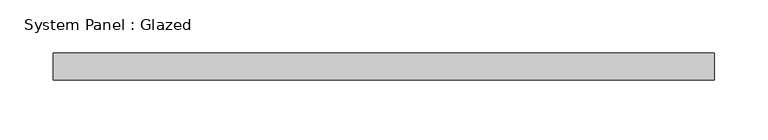
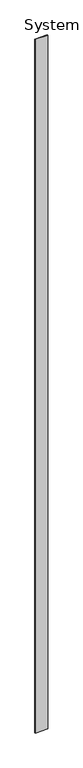
"""IFC4 building model written with IfcOpenShell, lengths in millimetres: plate geometry, System Panel : Glazed."""

from ifc_helpers import new_model, si_unit, origin, origin_with_axes, place, context, project, spatial, polyline, outline, extrude, source, transform, mapped, element, save


def system_panel_glazed_6238d1ea(model_context):
    return source(origin(), model_context, "Body", "SweptSolid", [
        extrude(outline(polyline([(311.15, 19.05), (-311.15, 19.05), (-311.15, 44.45), (311.15, 44.45), (311.15, 19.05)])), origin_with_axes(), (0.0, 0.0, 1.0), 36423.6),
    ])


if __name__ == "__main__":
    model = new_model("IFC4")
    model_context = context("Model", 3, world=origin())
    ifc_project = project(units=[si_unit("LENGTHUNIT", "METRE", prefix="MILLI")], contexts=[model_context])
    site = spatial("IfcSite", under=ifc_project)
    building = spatial("IfcBuilding", under=site)
    placement = place(None, origin())
    system_panel_glazed_shape = system_panel_glazed_6238d1ea(model_context)
    element("IfcPlate", 1, ObjectType="System Panel : Glazed", at=placement, inside=building, context=model_context, shape_type="MappedRepresentation", body=[
        mapped(system_panel_glazed_shape, transform((0.0, 0.0, 0.0), x_axis=(1.0, 0.0, 0.0), y_axis=(0.0, 1.0, 0.0), z_axis=(0.0, 0.0, 1.0))),
    ])
    save(model, "model.ifc")

# Revit data of these elements
# Type "System Panel : Glazed"
#   Construction Type Id = "GSP4R"
#   Analytic Construction = "1/8 in Pilkington single glazing"
#   Visual Light Transmittance = 0.9
#   Solar Heat Gain Coefficient = 0.86
#   Heat Transfer Coefficient (U) = 1.18115 BTU/(h·ft²·°F)
#   Define Thermal Properties by = 1
# Element 1 (IfcPlate, "System Panel : Glazed")
#   Materials on its faces: "Glass"
# Materials
#   "Glass": class "Glass", colour RGB 0 128 192, transparency 0.75, Description = "Soda Lime Glass", Cost = 0
